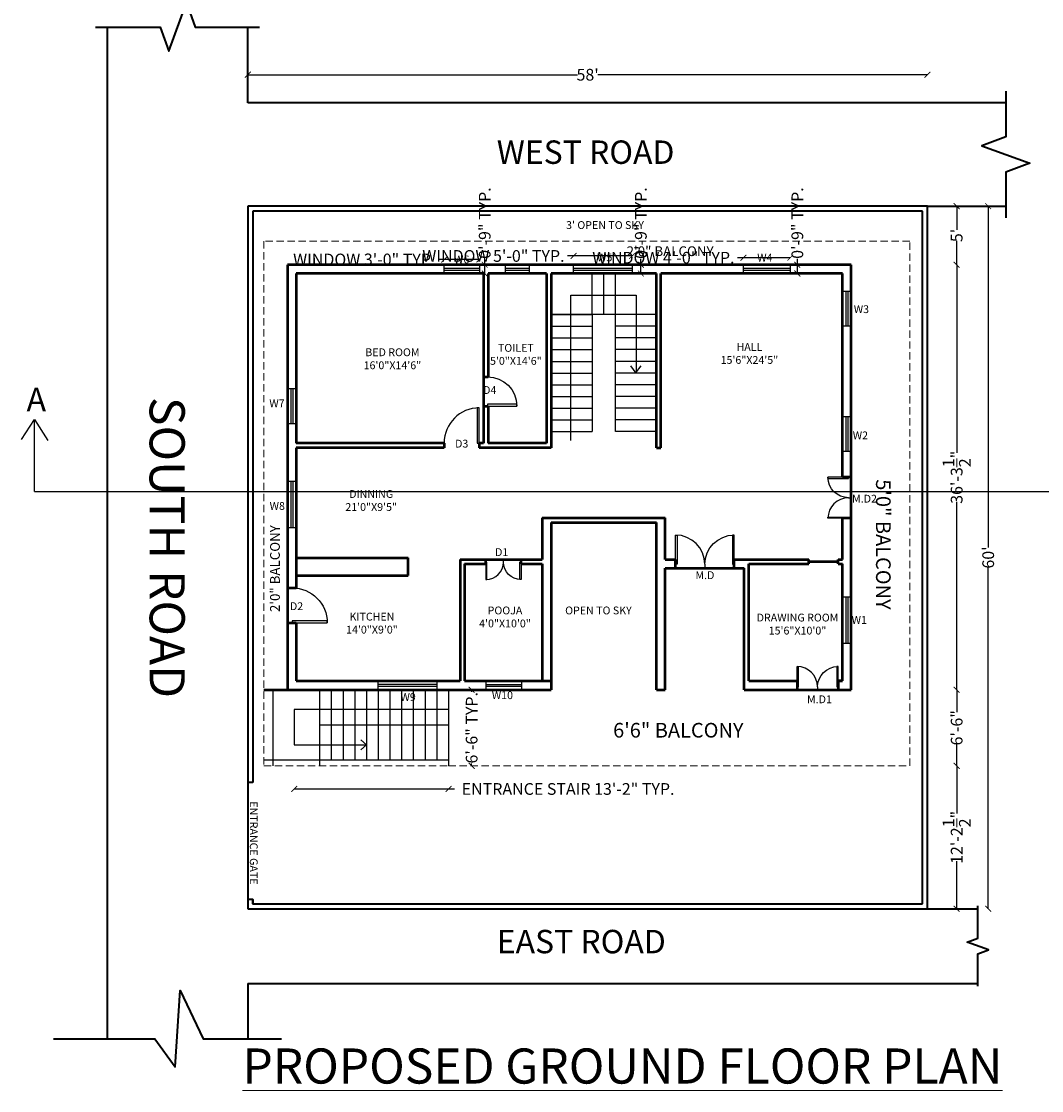
# Model space of a CAD drawing. Units: inches. Extents: x 626 to 5030, y -1681 to 1720.
# Tile 2 of 5: x 2115 to 3160, y 68 to 1163. Entities that reach past the tile are written whole.
import ezdxf

# ---------------------------------------------------------------- set-up
doc = ezdxf.new("R2010")
doc.units = ezdxf.units.IN
doc.header["$MEASUREMENT"] = 0
doc.linetypes.add('HIDDENX2', pattern=[0.75, 0.5, -0.25])
for name, color, linetype, lineweight in [('A-ANNO-DIMS', 2, 'Continuous', 18), ('A-ANNO-SYMB', 2, 'Continuous', 25), ('A-ANNO-TEXT', 7, 'Continuous', 18), ('A-AREA-IDEN', 3, 'Continuous', 18), ('A-DOOR', 4, 'Continuous', 25), ('A-FLOR-OVHD', 3, 'HIDDENX2', 18), ('A-FLOR-STRS', 3, 'Continuous', 25), ('A-GLAZ', 4, 'Continuous', 25), ('A-WALL', 7, 'Continuous', 50), ('C-PROP', 1, 'Continuous', 35)]:
    doc.layers.add(name, color=color, linetype=linetype, lineweight=lineweight)
doc.layers.add('windows', color=4, linetype='Continuous')
doc.styles.get("Standard").update_dxf_attribs({"font": 'arial.ttf'})
doc.dimstyles.get("Standard").update_dxf_attribs({"dimtxt": 12, "dimasz": 6, "dimexe": 0.18, "dimexo": 0.0625, "dimgap": 0.09, "dimtad": 0, "dimdec": 1, "dimzin": 0, "dimdsep": 46, "dimlunit": 4, "dimtxsty": 'Standard', "dimblk": 'ARCHTICK', "dimcen": 0.09, "dimse1": 1, "dimse2": 1, "dimclrt": 3, "dimadec": 0, "dimazin": 0, "dimtfac": 1, "dimtdec": 1, "dimtofl": 0, "dimtmove": 0, "dimatfit": 3, "dimfxl": 1, "dimtolj": 1, "dimtzin": 0, "dimarcsym": 0})

# ---------------------------------------------------------------- blocks, each defined once
blk = doc.blocks.new('_ArchTick')
at = {"color": 0, "linetype": 'ByBlock', "const_width": 0.15}
blk.add_lwpolyline([(-0.5, -0.5), (0.5, 0.5)], dxfattribs=at)
blk = doc.blocks.new('*D3')
at = {"layer": 'A-ANNO-DIMS', "color": 0, "lineweight": -2, "transparency": 16777216}
for p, q in [((2346.6, 1108.7), (2684.3, 1108.7)), ((3042.6, 1108.7), (2704.9, 1108.7))]:
    blk.add_line(p, q, dxfattribs=at)
at = {"layer": 'DEFPOINTS', "color": 0, "transparency": 16777216}
for p in [(3042.6, 1108.7), (2346.6, 974), (3042.6, 974)]:
    blk.add_point(p, dxfattribs=at)
at = {"layer": 'A-ANNO-DIMS', "color": 0, "lineweight": -2, "transparency": 16777216, "xscale": 6, "yscale": 6, "zscale": 6, "rotation": 180}
blk.add_blockref('_ArchTick', (2346.6, 1108.7), dxfattribs=at)
at = {"layer": 'A-ANNO-DIMS', "color": 0, "lineweight": -2, "transparency": 16777216, "xscale": 6, "yscale": 6, "zscale": 6}
blk.add_blockref('_ArchTick', (3042.6, 1108.7), dxfattribs=at)
at = {"layer": 'A-ANNO-DIMS', "color": 0, "transparency": 16777216, "insert": (2694.6, 1108.7), "char_height": 12, "attachment_point": 5}
blk.add_mtext("\\A1;58'", dxfattribs=at)
blk = doc.blocks.new('*D13')
at = {"layer": 'A-ANNO-DIMS', "color": 0, "lineweight": -2, "transparency": 16777216}
for p, q in [((3072.6, 914), (3072.6, 721.3)), ((3072.6, 478.5), (3072.6, 671.2))]:
    blk.add_line(p, q, dxfattribs=at)
at = {"layer": 'DEFPOINTS', "color": 0, "transparency": 16777216}
for p in [(2964.6, 914), (2657.1, 478.5), (3072.6, 478.5)]:
    blk.add_point(p, dxfattribs=at)
at = {"layer": 'A-ANNO-DIMS', "color": 0, "lineweight": -2, "transparency": 16777216, "xscale": 6, "yscale": 6, "zscale": 6}
for p, rotation in [((3072.6, 914), 90), ((3072.6, 478.5), 270)]:
    blk.add_blockref('_ArchTick', p, dxfattribs=dict(at, rotation=rotation))
at = {"layer": 'A-ANNO-DIMS', "color": 0, "transparency": 16777216, "insert": (3072.6, 696.2), "char_height": 12, "attachment_point": 5, "rotation": 90}
blk.add_mtext('\\A1;36\'-3{\\H1x;\\S1/2;}"', dxfattribs=at)
blk = doc.blocks.new('*D14')
at = {"layer": 'A-ANNO-DIMS', "color": 0, "lineweight": -2, "transparency": 16777216}
for p, q in [((3072.6, 974), (3072.6, 949.6)), ((3072.6, 914), (3072.6, 938.4))]:
    blk.add_line(p, q, dxfattribs=at)
at = {"layer": 'DEFPOINTS', "color": 0, "transparency": 16777216}
for p in [(2964.6, 974), (3072.6, 974), (2964.6, 914)]:
    blk.add_point(p, dxfattribs=at)
at = {"layer": 'A-ANNO-DIMS', "color": 0, "lineweight": -2, "transparency": 16777216, "xscale": 6, "yscale": 6, "zscale": 6}
for p, rotation in [((3072.6, 974), 90), ((3072.6, 914), 270)]:
    blk.add_blockref('_ArchTick', p, dxfattribs=dict(at, rotation=rotation))
at = {"layer": 'A-ANNO-DIMS', "color": 0, "transparency": 16777216, "insert": (3072.6, 944), "char_height": 12, "attachment_point": 5, "rotation": 90}
blk.add_mtext("\\A1;5'", dxfattribs=at)
blk = doc.blocks.new('*D15')
at = {"layer": 'A-ANNO-DIMS', "color": 0, "lineweight": -2, "transparency": 16777216}
for p, q in [((3072.6, 478.5), (3072.6, 455.6)), ((3072.6, 400.5), (3072.6, 423.4))]:
    blk.add_line(p, q, dxfattribs=at)
at = {"layer": 'DEFPOINTS', "color": 0, "transparency": 16777216}
for p in [(2964.6, 478.5), (2534.3, 400.5), (3072.6, 400.5)]:
    blk.add_point(p, dxfattribs=at)
at = {"layer": 'A-ANNO-DIMS', "color": 0, "lineweight": -2, "transparency": 16777216, "xscale": 6, "yscale": 6, "zscale": 6}
for p, rotation in [((3072.6, 478.5), 90), ((3072.6, 400.5), 270)]:
    blk.add_blockref('_ArchTick', p, dxfattribs=dict(at, rotation=rotation))
at = {"layer": 'A-ANNO-DIMS', "color": 0, "transparency": 16777216, "insert": (3072.6, 439.5), "char_height": 12, "attachment_point": 5, "rotation": 90}
blk.add_mtext('\\A1;6\'-6"', dxfattribs=at)
blk = doc.blocks.new('*D16')
at = {"layer": 'A-ANNO-DIMS', "color": 0, "lineweight": -2, "transparency": 16777216}
for p, q in [((3072.6, 400.5), (3072.6, 351.8)), ((3072.6, 254), (3072.6, 302.7))]:
    blk.add_line(p, q, dxfattribs=at)
at = {"layer": 'DEFPOINTS', "color": 0, "transparency": 16777216}
for p in [(3024.6, 400.5), (3024.6, 254), (3072.6, 254)]:
    blk.add_point(p, dxfattribs=at)
at = {"layer": 'A-ANNO-DIMS', "color": 0, "lineweight": -2, "transparency": 16777216, "xscale": 6, "yscale": 6, "zscale": 6}
for p, rotation in [((3072.6, 400.5), 90), ((3072.6, 254), 270)]:
    blk.add_blockref('_ArchTick', p, dxfattribs=dict(at, rotation=rotation))
at = {"layer": 'A-ANNO-DIMS', "color": 0, "transparency": 16777216, "insert": (3072.6, 327.2), "char_height": 12, "attachment_point": 5, "rotation": 90}
blk.add_mtext('\\A1;12\'-2{\\H1x;\\S1/2;}"', dxfattribs=at)
blk = doc.blocks.new('*D17')
at = {"layer": 'A-ANNO-DIMS', "color": 0, "lineweight": -2, "transparency": 16777216}
for p, q in [((3104.9, 974), (3104.9, 624.3)), ((3104.9, 254), (3104.9, 603.7))]:
    blk.add_line(p, q, dxfattribs=at)
at = {"layer": 'DEFPOINTS', "color": 0, "transparency": 16777216}
for p in [(3042.6, 974), (3042.6, 254), (3104.9, 254)]:
    blk.add_point(p, dxfattribs=at)
at = {"layer": 'A-ANNO-DIMS', "color": 0, "lineweight": -2, "transparency": 16777216, "xscale": 6, "yscale": 6, "zscale": 6}
for p, rotation in [((3104.9, 974), 90), ((3104.9, 254), 270)]:
    blk.add_blockref('_ArchTick', p, dxfattribs=dict(at, rotation=rotation))
at = {"layer": 'A-ANNO-DIMS', "color": 0, "transparency": 16777216, "insert": (3104.9, 614), "char_height": 12, "attachment_point": 5, "rotation": 90}
blk.add_mtext("\\A1;60'", dxfattribs=at)
blk = doc.blocks.new('*U19')
for p, q in [((0, 0), (0, -100)), ((750, 0), (750, -100))]:
    blk.add_line(p, q)
blk.add_lwpolyline([(0, 0), (0, 750), (43.75, 750), (43.75, 0)], close=True)
blk.add_arc((0, 0), 750, 0, 90)
blk = doc.blocks.new('*U20')
for p, q in [((0, 0), (0, 100)), ((750, 0), (750, 100))]:
    blk.add_line(p, q)
blk.add_lwpolyline([(0, 0), (0, -750), (43.75, -750), (43.75, 0)], close=True)
blk.add_arc((0, 0), 750, 270, 0)
blk = doc.blocks.new('*U22')
for p, q in [((-750, 0), (-750, -100)), ((0, 0), (0, -100))]:
    blk.add_line(p, q)
blk.add_lwpolyline([(0, 0), (0, 750), (-43.75, 750), (-43.75, 0)], close=True)
blk.add_arc((0, 0), 750, 90, 180)
blk = doc.blocks.new('*U21')
for p, q in [((0, 0), (0, -100)), ((750, 0), (750, -100))]:
    blk.add_line(p, q)
blk.add_lwpolyline([(0, 0), (0, 750), (43.75, 750), (43.75, 0)], close=True)
blk.add_arc((0, 0), 750, 0, 90)
blk = doc.blocks.new('W3')
at = {"layer": 'windows'}
for p, q in [((2120.1, 414.9), (2120.1, 378.9)), ((2122.1, 414.9), (2122.1, 378.9))]:
    blk.add_line(p, q, dxfattribs=at)
blk.add_lwpolyline([(2116.6, 414.9), (2125.6, 414.9), (2125.6, 378.9), (2116.6, 378.9)], close=True, dxfattribs=at)
blk = doc.blocks.new('W5')
at = {"layer": 'windows'}
for p, q in [((2038.2, 554.9), (2038.2, 494.9)), ((2040.2, 554.9), (2040.2, 494.9))]:
    blk.add_line(p, q, dxfattribs=at)
blk.add_lwpolyline([(2034.7, 554.9), (2043.7, 554.9), (2043.7, 494.9), (2034.7, 494.9)], close=True, dxfattribs=at)
blk = doc.blocks.new('WINDOW')
at = {"layer": 'windows'}
for p, q in [((173.6, 537.5), (173.6, 489.5)), ((175.6, 537.5), (175.6, 489.5))]:
    blk.add_line(p, q, dxfattribs=at)
blk.add_lwpolyline([(170.1, 537.5), (179.1, 537.5), (179.1, 489.5), (170.1, 489.5)], close=True, dxfattribs=at)
blk = doc.blocks.new('*U26')
for p, q in [((0, 0), (0, -100)), ((750, 0), (750, -100))]:
    blk.add_line(p, q)
blk.add_lwpolyline([(0, 0), (0, 750), (43.75, 750), (43.75, 0)], close=True)
blk.add_arc((0, 0), 750, 0, 90)
blk = doc.blocks.new('V1')
at = {"layer": 'windows'}
for p, q in [((3301.5, 317.5), (3301.5, 293.5)), ((3303.5, 317.5), (3303.5, 293.5))]:
    blk.add_line(p, q, dxfattribs=at)
blk.add_lwpolyline([(3298, 317.5), (3307, 317.5), (3307, 293.5), (3298, 293.5)], close=True, dxfattribs=at)
blk = doc.blocks.new('STAIR-INTERNAL')
for p, q in [((42, 120), (42, 162)), ((54, 120), (54, 162)), ((66, 120), (66, 162)), ((20.4, 139.7), (87.3, 139.7)), ((87.3, 139.7), (87.3, 60)), ((108, 120), (0, 120)), ((0, 120), (42, 120)), ((42, 120), (42, 0)), ((66, 0), (66, 120)), ((0, 108), (42, 108)), ((108, 108), (66, 108)), ((0, 96), (42, 96)), ((108, 96), (66, 96)), ((0, 84), (42, 84)), ((108, 84), (66, 84)), ((0, 72), (42, 72)), ((108, 72), (66, 72)), ((87.3, 60), (81.6, 67.5)), ((86.7, 60), (92.4, 67.5)), ((0, 60), (42, 60)), ((108, 60), (66, 60)), ((0, 48), (42, 48)), ((108, 48), (66, 48)), ((0, 36), (42, 36)), ((108, 36), (66, 36)), ((0, 24), (42, 24)), ((108, 24), (66, 24)), ((0, 12), (42, 12)), ((108, 12), (66, 12)), ((0, 0), (42, 0)), ((108, 0), (66, 0))]:
    blk.add_line(p, q)
blk = doc.blocks.new('STAIR-ENTRANCE')
for p, q in [((26.1, 78), (26.1, 0)), ((38.1, 78), (38.1, 6)), ((50.1, 78), (50.1, 6)), ((62.1, 78), (62.1, 6)), ((74.1, 78), (74.1, 6)), ((86.1, 78), (86.1, 6)), ((98.1, 78), (98.1, 6)), ((110.1, 78), (110.1, 6)), ((122.1, 78), (122.1, 6)), ((134.1, 78), (134.1, 6)), ((146.1, 78), (146.1, 6)), ((158.1, 78), (158.1, 0)), ((158.1, 57.8), (0, 57.8)), ((0, 57.8), (0, 21.7)), ((26.1, 42), (158.1, 42)), ((74.1, 21.7), (68.4, 26.8)), ((0, 21.7), (74.1, 21.7)), ((74.1, 21.7), (68.4, 16.5))]:
    blk.add_line(p, q)
blk = doc.blocks.new('*D54')
at = {"layer": 'A-ANNO-DIMS', "color": 0, "lineweight": -2, "transparency": 16777216}
for p, q in [((2547.8, 919.4), (2541.8, 919.4)), ((2583.8, 919.4), (2547.8, 919.4))]:
    blk.add_line(p, q, dxfattribs=at)
at = {"layer": 'DEFPOINTS', "color": 0, "transparency": 16777216}
for p in [(2547.8, 919.4), (2547.8, 914), (2583.8, 914)]:
    blk.add_point(p, dxfattribs=at)
at = {"layer": 'A-ANNO-DIMS', "color": 0, "lineweight": -2, "transparency": 16777216, "xscale": 6, "yscale": 6, "zscale": 6, "rotation": 180}
blk.add_blockref('_ArchTick', (2547.8, 919.4), dxfattribs=at)
at = {"layer": 'A-ANNO-DIMS', "color": 0, "lineweight": -2, "transparency": 16777216, "xscale": 6, "yscale": 6, "zscale": 6}
blk.add_blockref('_ArchTick', (2583.8, 919.4), dxfattribs=at)
at = {"layer": 'A-ANNO-DIMS', "color": 3, "transparency": 16777216, "insert": (2465.8, 919.4), "char_height": 12, "attachment_point": 5}
blk.add_mtext('\\A1;WINDOW 3\'-0" TYP.', dxfattribs=at)
blk = doc.blocks.new('*D55')
at = {"layer": 'A-ANNO-DIMS', "color": 0, "lineweight": -2, "transparency": 16777216}
for p, q in [((2589.2, 914), (2589.2, 920)), ((2589.2, 905), (2589.2, 914))]:
    blk.add_line(p, q, dxfattribs=at)
at = {"layer": 'DEFPOINTS', "color": 0, "transparency": 16777216}
for p in [(2583.8, 914), (2589.2, 914), (2583.8, 905)]:
    blk.add_point(p, dxfattribs=at)
at = {"layer": 'A-ANNO-DIMS', "color": 0, "lineweight": -2, "transparency": 16777216, "xscale": 6, "yscale": 6, "zscale": 6}
for p, rotation in [((2589.2, 914), 90), ((2589.2, 905), 270)]:
    blk.add_blockref('_ArchTick', p, dxfattribs=dict(at, rotation=rotation))
at = {"layer": 'A-ANNO-DIMS', "color": 3, "transparency": 16777216, "insert": (2589.2, 956.7), "char_height": 12, "attachment_point": 5, "rotation": 90}
blk.add_mtext('\\A1;0\'-9" TYP.', dxfattribs=at)
blk = doc.blocks.new('*D56')
at = {"layer": 'A-ANNO-DIMS', "color": 0, "lineweight": -2, "transparency": 16777216}
for p, q in [((2854.2, 921.2), (2848.2, 921.2)), ((2902.2, 921.2), (2854.2, 921.2))]:
    blk.add_line(p, q, dxfattribs=at)
at = {"layer": 'DEFPOINTS', "color": 0, "transparency": 16777216}
for p in [(2854.2, 921.2), (2854.2, 914), (2902.2, 914)]:
    blk.add_point(p, dxfattribs=at)
at = {"layer": 'A-ANNO-DIMS', "color": 0, "lineweight": -2, "transparency": 16777216, "xscale": 6, "yscale": 6, "zscale": 6, "rotation": 180}
blk.add_blockref('_ArchTick', (2854.2, 921.2), dxfattribs=at)
at = {"layer": 'A-ANNO-DIMS', "color": 0, "lineweight": -2, "transparency": 16777216, "xscale": 6, "yscale": 6, "zscale": 6}
blk.add_blockref('_ArchTick', (2902.2, 921.2), dxfattribs=at)
at = {"layer": 'A-ANNO-DIMS', "color": 3, "transparency": 16777216, "insert": (2772.2, 921.2), "char_height": 12, "attachment_point": 5}
blk.add_mtext('\\A1;WINDOW 4\'-0" TYP.', dxfattribs=at)
blk = doc.blocks.new('*D57')
at = {"layer": 'A-ANNO-DIMS', "color": 0, "lineweight": -2, "transparency": 16777216}
for p, q in [((2909.4, 914), (2909.4, 920)), ((2909.4, 905), (2909.4, 914))]:
    blk.add_line(p, q, dxfattribs=at)
at = {"layer": 'DEFPOINTS', "color": 0, "transparency": 16777216}
for p in [(2902.2, 914), (2909.4, 914), (2902.2, 905)]:
    blk.add_point(p, dxfattribs=at)
at = {"layer": 'A-ANNO-DIMS', "color": 0, "lineweight": -2, "transparency": 16777216, "xscale": 6, "yscale": 6, "zscale": 6}
for p, rotation in [((2909.4, 914), 90), ((2909.4, 905), 270)]:
    blk.add_blockref('_ArchTick', p, dxfattribs=dict(at, rotation=rotation))
at = {"layer": 'A-ANNO-DIMS', "color": 3, "transparency": 16777216, "insert": (2909.4, 956.7), "char_height": 12, "attachment_point": 5, "rotation": 90}
blk.add_mtext('\\A1;0\'-9" TYP.', dxfattribs=at)
blk = doc.blocks.new('*D58')
at = {"layer": 'A-ANNO-DIMS', "color": 0, "lineweight": -2, "transparency": 16777216}
for p, q in [((2680.1, 923), (2674.1, 923)), ((2740.1, 923), (2680.1, 923))]:
    blk.add_line(p, q, dxfattribs=at)
at = {"layer": 'DEFPOINTS', "color": 0, "transparency": 16777216}
for p in [(2680.1, 923), (2680.1, 914), (2740.1, 914)]:
    blk.add_point(p, dxfattribs=at)
at = {"layer": 'A-ANNO-DIMS', "color": 0, "lineweight": -2, "transparency": 16777216, "xscale": 6, "yscale": 6, "zscale": 6, "rotation": 180}
blk.add_blockref('_ArchTick', (2680.1, 923), dxfattribs=at)
at = {"layer": 'A-ANNO-DIMS', "color": 0, "lineweight": -2, "transparency": 16777216, "xscale": 6, "yscale": 6, "zscale": 6}
blk.add_blockref('_ArchTick', (2740.1, 923), dxfattribs=at)
at = {"layer": 'A-ANNO-DIMS', "color": 3, "transparency": 16777216, "insert": (2598.1, 923), "char_height": 12, "attachment_point": 5}
blk.add_mtext('\\A1;WINDOW 5\'-0" TYP.', dxfattribs=at)
blk = doc.blocks.new('*D59')
at = {"layer": 'A-ANNO-DIMS', "color": 0, "lineweight": -2, "transparency": 16777216}
for p, q in [((2749.1, 914), (2749.1, 920)), ((2749.1, 905), (2749.1, 914))]:
    blk.add_line(p, q, dxfattribs=at)
at = {"layer": 'DEFPOINTS', "color": 0, "transparency": 16777216}
for p in [(2740.1, 914), (2749.1, 914), (2740.1, 905)]:
    blk.add_point(p, dxfattribs=at)
at = {"layer": 'A-ANNO-DIMS', "color": 0, "lineweight": -2, "transparency": 16777216, "xscale": 6, "yscale": 6, "zscale": 6}
for p, rotation in [((2749.1, 914), 90), ((2749.1, 905), 270)]:
    blk.add_blockref('_ArchTick', p, dxfattribs=dict(at, rotation=rotation))
at = {"layer": 'A-ANNO-DIMS', "color": 3, "transparency": 16777216, "insert": (2749.1, 956.7), "char_height": 12, "attachment_point": 5, "rotation": 90}
blk.add_mtext('\\A1;0\'-9" TYP.', dxfattribs=at)
blk = doc.blocks.new('*D64')
at = {"layer": 'A-ANNO-DIMS', "color": 0, "lineweight": -2, "transparency": 16777216}
for p, q in [((2394, 376.8), (2552.1, 376.8)), ((2552.1, 376.8), (2558.1, 376.8))]:
    blk.add_line(p, q, dxfattribs=at)
at = {"layer": 'DEFPOINTS', "color": 0, "transparency": 16777216}
for p in [(2394, 400.5), (2552.1, 400.5), (2552.1, 376.8)]:
    blk.add_point(p, dxfattribs=at)
at = {"layer": 'A-ANNO-DIMS', "color": 0, "lineweight": -2, "transparency": 16777216, "xscale": 6, "yscale": 6, "zscale": 6, "rotation": 180}
blk.add_blockref('_ArchTick', (2394, 376.8), dxfattribs=at)
at = {"layer": 'A-ANNO-DIMS', "color": 0, "lineweight": -2, "transparency": 16777216, "xscale": 6, "yscale": 6, "zscale": 6}
blk.add_blockref('_ArchTick', (2552.1, 376.8), dxfattribs=at)
at = {"layer": 'A-ANNO-DIMS', "color": 3, "transparency": 16777216, "insert": (2674.6, 376.8), "char_height": 12, "attachment_point": 5}
blk.add_mtext('\\A1;ENTRANCE STAIR 13\'-2" TYP.', dxfattribs=at)
blk = doc.blocks.new('*D65')
at = {"layer": 'A-ANNO-DIMS', "color": 0, "lineweight": -2, "transparency": 16777216}
for p, q in [((2575.8, 478.5), (2575.8, 476.2)), ((2575.8, 400.5), (2575.8, 402.8))]:
    blk.add_line(p, q, dxfattribs=at)
at = {"layer": 'DEFPOINTS', "color": 0, "transparency": 16777216}
for p in [(2552.1, 478.5), (2575.8, 478.5), (2552.1, 400.5)]:
    blk.add_point(p, dxfattribs=at)
at = {"layer": 'A-ANNO-DIMS', "color": 0, "lineweight": -2, "transparency": 16777216, "xscale": 6, "yscale": 6, "zscale": 6}
for p, rotation in [((2575.8, 478.5), 90), ((2575.8, 400.5), 270)]:
    blk.add_blockref('_ArchTick', p, dxfattribs=dict(at, rotation=rotation))
at = {"layer": 'A-ANNO-DIMS', "color": 3, "transparency": 16777216, "insert": (2575.8, 439.5), "char_height": 12, "attachment_point": 5, "rotation": 90}
blk.add_mtext('\\A1;6\'-6" TYP.', dxfattribs=at)

msp = doc.modelspace()

# ---------------------------------------------------------------- linework, layer by layer
at = {"layer": 'A-ANNO-SYMB'}
for q in [(2128.1, 755.5), (3966.1, 681.5)]:
    msp.add_line((2128.1, 681.5), q, dxfattribs=at)
msp.add_lwpolyline([(2114.6, 735), (2128.1, 755.5), (2141.6, 734)], dxfattribs=at)
at = {"layer": 'A-FLOR-OVHD', "ltscale": 15}
for p, q in [((2363.1, 938), (2363.1, 400.5)), ((3024.6, 938), (2363.1, 938)), ((3024.6, 400.5), (3024.6, 938)), ((2363.1, 400.5), (2552.1, 400.5)), ((2552.1, 400.5), (3024.6, 400.5))]:
    msp.add_line(p, q, dxfattribs=at)
at = {"layer": 'A-FLOR-STRS'}
for p, q in [((2677.49, 733.76), (2677.49, 882.68)), ((2372.1, 478.5), (2372.1, 400.5)), ((2363.1, 406.5), (2552.1, 406.5))]:
    msp.add_line(p, q, dxfattribs=at)
at = {"layer": 'A-WALL'}
for p, q in [((2964.6, 914), (2387.1, 914)), ((2387.1, 914), (2387.1, 478.5)), ((2964.6, 478.5), (2964.6, 914)), ((2396.1, 905), (2396.1, 731)), ((2588.1, 905), (2396.1, 905)), ((2588.1, 905), (2588.1, 799.22)), ((2592.6, 905), (2592.6, 799.22)), ((2652.6, 905), (2592.6, 905)), ((2652.6, 905), (2652.6, 731)), ((2657.1, 905), (2657.1, 726.5)), ((2765.1, 905), (2657.1, 905)), ((2765.1, 726.5), (2765.1, 905)), ((2955.6, 905), (2769.6, 905)), ((2769.6, 726.5), (2769.6, 905)), ((2955.6, 696.5), (2955.6, 905)), ((2588.1, 799.22), (2592.6, 799.22)), ((2588.1, 799.22), (2588.1, 731)), ((2588.1, 769.22), (2592.6, 769.22)), ((2592.6, 769.22), (2592.6, 731)), ((2547.6, 731), (2396.1, 731)), ((2396.1, 726.5), (2396.1, 582.92)), ((2547.6, 726.5), (2396.1, 726.5)), ((2547.6, 731), (2547.6, 726.5)), ((2588.1, 731), (2583.6, 731)), ((2583.6, 731), (2583.6, 726.5)), ((2588.1, 731), (2583.6, 731)), ((2657.1, 726.5), (2583.6, 726.5)), ((2652.6, 731), (2592.6, 731)), ((2765.1, 726.5), (2769.6, 726.5)), ((2955.6, 696.5), (2964.6, 696.5)), ((2648.1, 654.5), (2648.1, 612)), ((2648.1, 654.5), (2774.1, 654.5)), ((2657.1, 650), (2657.1, 478.5)), ((2657.1, 650), (2765.1, 650)), ((2765.1, 478.5), (2765.1, 650)), ((2774.1, 612), (2774.1, 654.5)), ((2955.6, 612), (2955.6, 654.5)), ((2955.6, 654.5), (2964.6, 654.5)), ((2396.1, 613.5), (2510.74, 613.5)), ((2510.74, 595.5), (2510.74, 613.5)), ((2564.1, 612), (2590.35, 612)), ((2564.1, 612), (2564.1, 487.5)), ((2564.1, 612), (2648.1, 612)), ((2568.6, 607.5), (2590.35, 607.5)), ((2568.6, 607.5), (2568.6, 487.5)), ((2590.35, 607.5), (2590.35, 612)), ((2626.35, 607.5), (2626.35, 612)), ((2626.35, 607.5), (2648.1, 607.5)), ((2648.1, 607.5), (2648.1, 487.5)), ((2774.1, 612), (2784.6, 612)), ((2774.1, 478.5), (2774.1, 603)), ((2774.1, 603), (2855.1, 603)), ((2784.6, 603), (2784.6, 612)), ((2844.6, 603), (2844.6, 612)), ((2844.6, 612), (2921.1, 612)), ((2844.6, 603), (2855.1, 603)), ((2855.1, 478.5), (2855.1, 603)), ((2859.6, 487.5), (2859.6, 607.5)), ((2859.6, 607.5), (2921.1, 607.5)), ((2921.1, 607.5), (2921.1, 612)), ((2921.1, 609.75), (2951.1, 609.75)), ((2951.1, 607.5), (2951.1, 612)), ((2951.1, 612), (2955.6, 612)), ((2951.1, 607.5), (2955.6, 607.5)), ((2955.6, 487.5), (2955.6, 607.5)), ((2396.1, 595.5), (2510.74, 595.5)), ((2387.1, 582.92), (2396.1, 582.92)), ((2387.1, 546.92), (2396.1, 546.92)), ((2396.1, 546.92), (2396.1, 487.5)), ((2396.1, 487.5), (2564.1, 487.5)), ((2568.6, 487.5), (2657.1, 487.5)), ((2859.6, 487.5), (2909.1, 487.5)), ((2909.1, 487.5), (2909.1, 478.5)), ((2955.6, 487.5), (2951.1, 487.5)), ((2951.1, 487.5), (2951.1, 478.5)), ((2951.1, 487.5), (2955.6, 487.5)), ((2363.1, 478.5), (2657.1, 478.5)), ((2765.1, 478.5), (2774.1, 478.5)), ((2855.1, 478.5), (2964.6, 478.5)), ((2951.1, 478.5), (2964.6, 478.5))]:
    msp.add_line(p, q, dxfattribs=at)
at = {"layer": 'C-PROP'}
for p, q in [((2202.6, 1157.57), (2202.6, 120.64)), ((2346.6, 1079.84), (2346.6, 1157.57)), ((3122.95, 1079.84), (2346.6, 1079.84)), ((3042.6, 974), (2346.6, 974)), ((2346.6, 974), (2346.6, 254)), ((3037.6, 969), (2351.6, 969)), ((2351.6, 969), (2351.6, 383.5)), ((3037.6, 259), (3037.6, 969)), ((3042.6, 254), (3042.6, 974)), ((3042.6, 974), (3122.95, 974)), ((2351.6, 383.5), (2346.6, 383.5)), ((2346.6, 254), (3042.6, 254)), ((2351.6, 259), (3037.6, 259)), ((3042.6, 254), (3094.18, 254)), ((2346.6, 177.61), (3094.18, 177.61)), ((2346.6, 177.61), (2346.6, 120.64))]:
    msp.add_line(p, q, dxfattribs=at)
for points in [[(2190.6, 1157.57), (2256.6, 1157.57), (2265.6, 1132.84), (2283.6, 1182.29), (2292.6, 1157.57), (2358.6, 1157.57)], [(3122.95, 1091.84), (3122.95, 1044.92), (3098.22, 1035.92), (3147.67, 1017.92), (3122.95, 1008.92), (3122.95, 962)], [(2351.6, 263.5), (2351.6, 259), (2351.6, 263.5), (2346.6, 263.5)], [(3094.18, 174.61), (3094.18, 207.8), (3105.17, 211.8), (3083.19, 219.8), (3094.18, 223.8), (3094.18, 257)], [(2147.34, 120.64), (2251.36, 120.64), (2272.1, 92.06), (2277.1, 170.16), (2300.64, 120.64), (2380.97, 120.64)]]:
    msp.add_lwpolyline(points, dxfattribs=at)

# ---------------------------------------------------------------- block references
at = {"layer": 'A-DOOR'}
for name, p, xscale, yscale, zscale, rotation in [('*U21', (2592.1, 769.22), -0.04, 0.04, 0.04, 270), ('*U26', (2961.8, 696.25), -0.0279999999999999, 0.0279999999999999, 0.0279999999999999, 90), ('*U26', (2961.8, 654.25), 0.0279999999999999, 0.0279999999999999, 0.0279999999999999, 90), ('*U21', (2391.9, 546.92), -0.048, 0.048, 0.048, 270)]:
    msp.add_blockref(name, p, dxfattribs=dict(at, xscale=xscale, yscale=yscale, zscale=zscale, rotation=rotation))
for name, p, xscale, yscale, zscale in [('*U22', (2583.6, 731.3), 0.0479999999999998, 0.0479999999999998, 0.0479999999999998), ('*U19', (2784.6, 607), 0.0399999999999999, 0.0399999999999999, 0.0399999999999999), ('*U19', (2844.6, 607), -0.0399999999999999, 0.0399999999999999, 0.0399999999999999), ('*U20', (2590.35, 609.35), 0.0239999999999999, 0.0239999999999999, 0.0239999999999999), ('*U20', (2626.35, 609.35), -0.0239999999999999, 0.0239999999999999, 0.0239999999999999), ('*U26', (2909.1, 481.3), 0.0279999999999999, 0.0279999999999999, 0.0279999999999999), ('*U26', (2951.1, 481.3), -0.0279999999999999, 0.0279999999999999, 0.0279999999999999)]:
    msp.add_blockref(name, p, dxfattribs=dict(at, xscale=xscale, yscale=yscale, zscale=zscale))
at = {"layer": 'A-FLOR-STRS'}
for name, p in [('STAIR-INTERNAL', (2657.1, 743)), ('STAIR-ENTRANCE', (2393.96, 400.5))]:
    msp.add_blockref(name, p, dxfattribs=at)
at = {"layer": 'A-GLAZ', "rotation": 90}
for name, p in [('W3', (2962.68, -1211.6)), ('V1', (2928.13, -2393)), ('W5', (3235.02, -1129.66)), ('WINDOW', (3391.69, 734.95)), ('W5', (3034.98, -1556.16)), ('W3', (3005.6, -1638.1))]:
    msp.add_blockref(name, p, dxfattribs=at)
at = {"layer": 'A-GLAZ'}
for name, p in [('W3', (839.01, 472.03)), ('W3', (270.51, 372.13)), ('W3', (839.01, 343.63)), ('WINDOW', (2217.05, 154.8)), ('WINDOW', (2785.55, 36.23))]:
    msp.add_blockref(name, p, dxfattribs=at)

# ---------------------------------------------------------------- texts
at = {"layer": 'A-ANNO-SYMB', "insert": (2113.97, 787.94), "char_height": 24, "attachment_point": 1}
msp.add_mtext_dynamic_manual_height_columns('\\pxqc;A', width=31.8381, gutter_width=1, heights=[0], dxfattribs=at)
at = {"layer": 'A-ANNO-TEXT', "attachment_point": 1}
for s, width, insert, char_height in [('WEST ROAD', 299.1904, (2601.53, 1041.35), 24), ("\\pxqc;3' OPEN TO SKY", 100.5461, (2662.12, 958.66), 8), ('\\pxqc;2\'0" BALCONY', 192.2401, (2682.95, 932.85), 10), ('\\pxqc;W6', 31.8381, (2549.73, 923.36), 8), ('\\pxqc;W5', 31.8381, (2696.22, 925.47), 8), ('\\pxqc;W4', 31.8381, (2860.21, 925.19), 8), ('\\pxqc;W3', 31.8381, (2959.12, 872.44), 8), ('\\pxqc;D4', 38.7401, (2574.98, 789.58), 8), ('\\pxqc;W7', 31.8381, (2360.47, 775.95), 8), ('\\pxqc;D3', 38.7401, (2546.26, 734.67), 8), ('\\pxqc;W2', 31.8381, (2958.07, 743.15), 8), ('\\pxqc;W8', 31.8381, (2360.77, 670.79), 8), ('\\pxqc;M.D2', 100.5461, (2927.94, 678.26), 8), ('\\pxqc;D1', 38.7401, (2587.17, 623.48), 8), ('\\pxqc;M.D', 100.5461, (2764.45, 599.88), 8), ('\\pxqc;D2', 38.7401, (2377.05, 568.1), 8), ('\\pxqc;OPEN TO SKY', 100.5461, (2655.4, 563.73), 8), ('\\pxqc;W1', 31.8381, (2956.94, 554.02), 8), ('\\pxqc;W9', 31.8381, (2494.83, 475), 8), ('\\pxqc;W10', 31.8381, (2591.39, 476.86), 8), ('\\pxqc;M.D1', 100.5461, (2881.77, 472.69), 8), ('\\pxqc;6\'6" BALCONY', 192.2401, (2691.38, 444.5), 15), ('EAST ROAD', 299.1904, (2601.53, 232.41), 24), ('\\pxt25;{\\LPROPOSED GROUND FLOOR PLAN}', 851.5031, (2341.03, 110.9), 36)]:
    msp.add_mtext_dynamic_manual_height_columns(s, width=width, gutter_width=1, heights=[0], dxfattribs=dict(at, insert=insert, char_height=char_height))
for s, width, insert, char_height, rotation in [('SOUTH ROAD', 372.8618, (2281.96, 778.49), 36, 270), ('\\pxqc;5\'0" BALCONY', 192.2401, (3004.98, 723.46), 15, 270), ('\\pxqc;2\'0" BALCONY', 192.2401, (2369.33, 506.48), 10, 90), ('\\pxqc;ENTRANCE GATE', 101.9862, (2356.6, 372.5), 8, 270)]:
    msp.add_mtext_dynamic_manual_height_columns(s, width=width, gutter_width=1, heights=[0], dxfattribs=dict(at, insert=insert, char_height=char_height, rotation=rotation))
at = {"layer": 'A-AREA-IDEN', "char_height": 8, "attachment_point": 1}
for s, insert in [('\\pxqc;TOILET\\P5\'0"X14\'6"', (2570.83, 832.81)), ('\\pxqc;HALL\\P15\'6"X24\'5"', (2810.05, 833.77)), ('\\pxqc;BED ROOM\\P16\'0"X14\'6"', (2444.37, 828.3)), ('\\pxqc;DINNING\\P21\'0"X9\'5"', (2422.63, 683.07)), ('\\pxqc;POOJA\\P4\'0"X10\'0"', (2559.7, 563.73)), ('\\pxqc;KITCHEN\\P14\'0"X9\'0"', (2423.41, 557.39)), ('\\pxqc;DRAWING ROOM\\P15\'6"X10\'0"', (2859.3, 556.42))]:
    msp.add_mtext_dynamic_manual_height_columns(s, width=100.5461, gutter_width=1, heights=[0], dxfattribs=dict(at, insert=insert))

# ---------------------------------------------------------------- dimensions: what is measured, and where the dimension line sits
at = {"layer": 'A-ANNO-DIMS'}
dim = msp.add_linear_dim(base=(3042.6, 1108.69), p1=(2346.6, 974), p2=(3042.6, 974), dimstyle='Standard', override={"dimclrd": 0, "dimclre": 0, "dimclrt": 0}, dxfattribs=at)
dim.commit()
dim.dimension.update_dxf_attribs({"geometry": '*D3', "text_midpoint": (2694.6, 1108.69)})
for base, p1, p2, angle, text, picture, middle in [((2589.2, 914), (2583.8, 905), (2583.8, 914), 90, '<> TYP.', '*D55', (2589.2, 956.66)), ((2749.14, 914), (2740.14, 905), (2740.14, 914), 90, '<> TYP.', '*D59', (2749.14, 956.66)), ((2909.37, 914), (2902.17, 905), (2902.17, 914), 90, '<> TYP.', '*D57', (2909.37, 956.66)), ((2547.8, 919.4), (2583.8, 914), (2547.8, 914), 180, 'WINDOW <> TYP.', '*D54', (2465.79, 919.4)), ((2680.14, 923), (2740.14, 914), (2680.14, 914), 180, 'WINDOW <> TYP.', '*D58', (2598.13, 923)), ((2854.17, 921.2), (2902.17, 914), (2854.17, 914), 180, 'WINDOW <> TYP.', '*D56', (2772.15, 921.2)), ((2575.83, 478.5), (2552.1, 400.5), (2552.1, 478.5), 90, '<> TYP.', '*D65', (2575.83, 439.5))]:
    dim = msp.add_linear_dim(base=base, p1=p1, p2=p2, angle=angle, text=text, dimstyle='Standard', override={"dimdec": 1, "dimrnd": 0, "dimzin": 1, "dimlunit": 4, "dimfrac": 2}, dxfattribs=at)
    dim.commit()
    dim.dimension.update_dxf_attribs({"geometry": picture, "text_midpoint": middle})
for base, p1, p2, picture, middle in [((3072.56, 974), (2964.6, 914), (2964.6, 974), '*D14', (3072.56, 944)), ((3104.9, 254), (3042.6, 974), (3042.6, 254), '*D17', (3104.9, 614)), ((3072.56, 478.5), (2964.6, 914), (2657.1, 478.5), '*D13', (3072.56, 696.25)), ((3072.56, 400.5), (2964.6, 478.5), (2534.32, 400.5), '*D15', (3072.56, 439.5)), ((3072.56, 254), (3024.6, 400.5), (3024.6, 254), '*D16', (3072.56, 327.25))]:
    dim = msp.add_linear_dim(base=base, p1=p1, p2=p2, angle=90, dimstyle='Standard', override={"dimclrd": 0, "dimclre": 0, "dimclrt": 0}, dxfattribs=at)
    dim.commit()
    dim.dimension.update_dxf_attribs({"geometry": picture, "text_midpoint": middle})
dim = msp.add_linear_dim(base=(2552.1, 376.78), p1=(2393.96, 400.5), p2=(2552.1, 400.5), text='ENTRANCE STAIR <> TYP.', dimstyle='Standard', override={"dimdec": 1, "dimrnd": 0, "dimzin": 1, "dimlunit": 4, "dimfrac": 2}, dxfattribs=at)
dim.commit()
dim.dimension.update_dxf_attribs({"geometry": '*D64', "text_midpoint": (2674.56, 376.78)})

doc.saveas('drawing.dxf')
